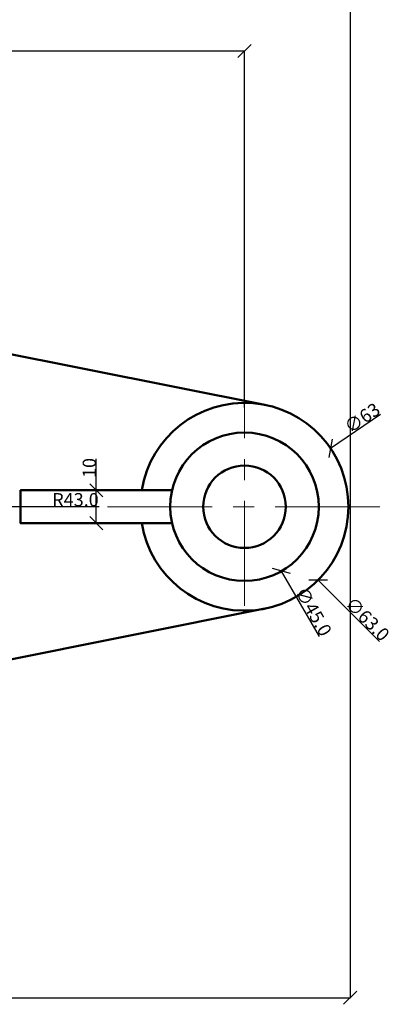
# Model space of a CAD drawing. Units: millimetres. Extents: x 263 to 611, y 50 to 522.
# Tile 4 of 5: x 478 to 591, y 50 to 349. Entities that reach past the tile are written whole.
import ezdxf

# ---------------------------------------------------------------- set-up
doc = ezdxf.new("R2010")
doc.units = ezdxf.units.MM
doc.header["$MEASUREMENT"] = 0
doc.linetypes.add('CENTER', pattern=[50.8, 31.75, -6.35, 6.35, -6.35])
for name, color, linetype, lineweight in [('M-CNTR', 1, 'CENTER', 18), ('M-DIMS', 2, 'Continuous', 25), ('M-OUTL', 7, 'Continuous', 50)]:
    doc.layers.add(name, color=color, linetype=linetype, lineweight=lineweight)
doc.styles.get("Standard").update_dxf_attribs({"font": 'arial.ttf'})
doc.dimstyles.get("Standard").update_dxf_attribs({"dimtxt": 4, "dimasz": 4, "dimexe": 0.18, "dimexo": 0.0625, "dimgap": 0.09, "dimtad": 1, "dimdec": 0, "dimzin": 0, "dimdsep": 46, "dimtxsty": 'Standard', "dimblk": 'OBLIQUE', "dimcen": 0.09, "dimclre": 251, "dimadec": 0, "dimazin": 0, "dimtfac": 1, "dimtdec": 0, "dimtofl": 0, "dimtmove": 0, "dimatfit": 3, "dimfxl": 1, "dimtolj": 1, "dimtzin": 0, "dimarcsym": 0})

# ---------------------------------------------------------------- blocks, each defined once
blk = doc.blocks.new('_Oblique')
at = {"color": 0, "linetype": 'ByBlock', "lineweight": -2}
blk.add_line((-0.5, -0.5), (0.5, 0.5), dxfattribs=at)
blk = doc.blocks.new('*D18')
at = {"layer": 'Defpoints', "color": 0, "transparency": 16777216}
for p in [(546.1, 339.25), (546.1, 231.08), (311.1, 223.08)]:
    blk.add_point(p, dxfattribs=at)
at = {"layer": 'M-DIMS', "color": 0, "lineweight": -2, "transparency": 16777216}
for p, q in [((311.1, 223.14), (311.1, 339.43)), ((311.1, 339.25), (546.1, 339.25)), ((546.1, 231.14), (546.1, 339.43))]:
    blk.add_line(p, q, dxfattribs=at)
at = {"layer": 'M-DIMS', "color": 0, "lineweight": -2, "transparency": 16777216, "xscale": 4, "yscale": 4, "zscale": 4, "rotation": 180}
blk.add_blockref('_Oblique', (311.1, 339.25), dxfattribs=at)
at = {"layer": 'M-DIMS', "color": 0, "lineweight": -2, "transparency": 16777216, "xscale": 4, "yscale": 4, "zscale": 4}
blk.add_blockref('_Oblique', (546.1, 339.25), dxfattribs=at)
at = {"layer": 'M-DIMS', "color": 0, "transparency": 16777216, "insert": (428.6, 341.39), "char_height": 4, "attachment_point": 5}
blk.add_mtext('\\A1;235', dxfattribs=at)
blk = doc.blocks.new('*D28')
at = {"layer": 'Defpoints', "color": 0, "transparency": 16777216}
for p in [(501.21, 206.08), (501.21, 206.08), (501.21, 196.08)]:
    blk.add_point(p, dxfattribs=at)
at = {"layer": 'M-DIMS', "color": 0, "lineweight": -2, "transparency": 16777216}
for p, q in [((501.21, 206.08), (501.21, 215.6)), ((501.15, 206.08), (501.03, 206.08)), ((501.21, 196.08), (501.21, 206.08)), ((501.15, 196.08), (501.03, 196.08))]:
    blk.add_line(p, q, dxfattribs=at)
at = {"layer": 'M-DIMS', "color": 0, "lineweight": -2, "transparency": 16777216, "xscale": 4, "yscale": 4, "zscale": 4}
for p, rotation in [((501.21, 206.08), 90), ((501.21, 196.08), 270)]:
    blk.add_blockref('_Oblique', p, dxfattribs=dict(at, rotation=rotation))
at = {"layer": 'M-DIMS', "color": 0, "transparency": 16777216, "insert": (499.08, 212.84), "char_height": 4, "attachment_point": 5, "rotation": 90}
blk.add_mtext('\\A1;10', dxfattribs=at)
blk = doc.blocks.new('*D34')
at = {"layer": 'Defpoints', "color": 0, "transparency": 16777216}
for p in [(572.16, 218.78), (520.04, 183.39)]:
    blk.add_point(p, dxfattribs=at)
at = {"layer": 'M-DIMS', "color": 0, "lineweight": -2, "transparency": 16777216}
for p, q in [((587.27, 229.04), (572.16, 218.78)), ((546.01, 201.08), (546.19, 201.08)), ((546.1, 200.99), (546.1, 201.17))]:
    blk.add_line(p, q, dxfattribs=at)
at = {"layer": 'M-DIMS', "color": 0, "lineweight": -2, "transparency": 16777216, "xscale": 4, "yscale": 4, "zscale": 4, "rotation": 214.179634482308}
blk.add_blockref('_Oblique', (572.16, 218.78), dxfattribs=at)
at = {"layer": 'M-DIMS', "color": 0, "transparency": 16777216, "insert": (581.76, 228.01), "char_height": 4, "attachment_point": 5, "rotation": 34.1796}
blk.add_mtext('\\A1;∅63', dxfattribs=at)
blk = doc.blocks.new('*D53')
at = {"layer": 'Defpoints', "color": 0, "transparency": 16777216}
for p in [(578.1, 423.27), (311.1, 383.27), (578.1, 52.26)]:
    blk.add_point(p, dxfattribs=at)
at = {"layer": 'M-DIMS', "color": 251, "lineweight": -2, "transparency": 16777216}
for p, q in [((578.1, 423.21), (578.1, 52.08)), ((311.1, 383.21), (311.1, 52.08))]:
    blk.add_line(p, q, dxfattribs=at)
at = {"layer": 'M-DIMS', "color": 0, "lineweight": -2, "transparency": 16777216}
blk.add_line((311.1, 52.26), (578.1, 52.26), dxfattribs=at)
at = {"layer": 'M-DIMS', "color": 0, "lineweight": -2, "transparency": 16777216, "xscale": 4, "yscale": 4, "zscale": 4, "rotation": 180}
blk.add_blockref('_Oblique', (311.1, 52.26), dxfattribs=at)
at = {"layer": 'M-DIMS', "color": 0, "lineweight": -2, "transparency": 16777216, "xscale": 4, "yscale": 4, "zscale": 4}
blk.add_blockref('_Oblique', (578.1, 52.26), dxfattribs=at)
at = {"layer": 'M-DIMS', "color": 0, "transparency": 16777216, "insert": (444.6, 54.39), "char_height": 4, "attachment_point": 5}
blk.add_mtext('\\A1;267.0', dxfattribs=at)
blk = doc.blocks.new('*D70')
at = {"layer": 'Defpoints', "color": 0, "transparency": 16777216}
for p in [(426.1, 201.08), (469.1, 201.08)]:
    blk.add_point(p, dxfattribs=at)
at = {"layer": 'M-DIMS', "color": 251, "lineweight": -2, "transparency": 16777216}
for p, q in [((426.01, 201.08), (426.19, 201.08)), ((426.1, 200.99), (426.1, 201.17))]:
    blk.add_line(p, q, dxfattribs=at)
at = {"layer": 'M-DIMS', "color": 0, "lineweight": -2, "transparency": 16777216}
blk.add_line((502.09, 201.08), (469.1, 201.08), dxfattribs=at)
at = {"layer": 'M-DIMS', "color": 0, "lineweight": -2, "transparency": 16777216, "xscale": 4, "yscale": 4, "zscale": 4, "rotation": 180.0006262561947}
blk.add_blockref('_Oblique', (469.1, 201.08), dxfattribs=at)
at = {"layer": 'M-DIMS', "color": 0, "transparency": 16777216, "insert": (494.9, 203.22), "char_height": 4, "attachment_point": 5, "rotation": 0.0006}
blk.add_mtext('\\A1;R43.0', dxfattribs=at)
blk = doc.blocks.new('*D72')
at = {"layer": 'Defpoints', "color": 0, "transparency": 16777216}
for p in [(523.82, 223.35), (568.38, 178.82)]:
    blk.add_point(p, dxfattribs=at)
at = {"layer": 'M-DIMS', "color": 251, "lineweight": -2, "transparency": 16777216}
for p, q in [((546.01, 201.08), (546.19, 201.08)), ((546.1, 200.99), (546.1, 201.17))]:
    blk.add_line(p, q, dxfattribs=at)
at = {"layer": 'M-DIMS', "color": 0, "lineweight": -2, "transparency": 16777216}
blk.add_line((587.03, 160.19), (568.38, 178.82), dxfattribs=at)
at = {"layer": 'M-DIMS', "color": 0, "lineweight": -2, "transparency": 16777216, "xscale": 4, "yscale": 4, "zscale": 4, "rotation": 135.0252345814981}
blk.add_blockref('_Oblique', (568.38, 178.82), dxfattribs=at)
at = {"layer": 'M-DIMS', "color": 0, "transparency": 16777216, "insert": (583.34, 167.05), "char_height": 4, "attachment_point": 5, "rotation": 315.0252}
blk.add_mtext('\\A1;∅63.0', dxfattribs=at)
blk = doc.blocks.new('*D73')
at = {"layer": 'Defpoints', "color": 0, "transparency": 16777216}
for p in [(534.85, 220.57), (557.35, 181.59)]:
    blk.add_point(p, dxfattribs=at)
at = {"layer": 'M-DIMS', "color": 251, "lineweight": -2, "transparency": 16777216}
for p, q in [((546.01, 201.08), (546.19, 201.08)), ((546.1, 200.99), (546.1, 201.17))]:
    blk.add_line(p, q, dxfattribs=at)
at = {"layer": 'M-DIMS', "color": 0, "lineweight": -2, "transparency": 16777216}
blk.add_line((568.8, 161.75), (557.35, 181.59), dxfattribs=at)
at = {"layer": 'M-DIMS', "color": 0, "lineweight": -2, "transparency": 16777216, "xscale": 4, "yscale": 4, "zscale": 4, "rotation": 119.9949843356095}
blk.add_blockref('_Oblique', (557.35, 181.59), dxfattribs=at)
at = {"layer": 'M-DIMS', "color": 0, "transparency": 16777216, "insert": (567.02, 169.33), "char_height": 4, "attachment_point": 5, "rotation": 299.995}
blk.add_mtext('\\A1;∅45.0', dxfattribs=at)

msp = doc.modelspace()

# ---------------------------------------------------------------- linework, layer by layer
at = {"layer": 'M-CNTR'}
for p, q in [((546.0988, 171.0815), (546.0988, 231.0815)), ((587.1329, 201.0815), (311.0988, 201.0815))]:
    msp.add_line(p, q, dxfattribs=at)
at = {"layer": 'M-OUTL'}
for p, q in [((552.2661, 231.9719), (436.0988, 255.1648)), ((552.2661, 170.1912), (436.0988, 146.9983))]:
    msp.add_line(p, q, dxfattribs=at)
msp.add_lwpolyline([(524.1614, 196.0815), (478.2588, 196.0815), (478.2588, 206.0815), (524.1614, 206.0815)], dxfattribs=at)
for radius in [22.5, 12.5]:
    msp.add_circle((546.0988, 201.0815), radius, dxfattribs=at)
msp.add_arc((546.0988, 201.0815), 31.5, 189.133198, 170.866802, dxfattribs=at)

# ---------------------------------------------------------------- dimensions: what is measured, and where the dimension line sits
at = {"layer": 'M-DIMS'}
for base, p1, p2, override, picture, middle in [((578.0988, 52.2557), (311.0988, 383.2727), (578.0988, 423.2727), {"dimdec": 1, "dimlfac": 1, "dimrnd": 0, "dimzin": 0, "dimdsep": 46, "dimlunit": 2}, '*D53', (444.5988, 54.388)), ((546.0988, 339.2528), (311.0988, 223.0815), (546.0988, 231.0815), {"dimclrd": 0, "dimclre": 0, "dimclrt": 0}, '*D18', (428.5988, 341.3864))]:
    dim = msp.add_linear_dim(base=base, p1=p1, p2=p2, dimstyle='Standard', override=override, dxfattribs=at)
    dim.commit()
    dim.dimension.update_dxf_attribs({"geometry": picture, "text_midpoint": middle})
dim = msp.add_diameter_dim_2p(p1=(520.0395, 183.3852), p2=(572.1582, 218.7779), dimstyle='Standard', override={"dimclrd": 0, "dimclre": 0, "dimclrt": 0}, dxfattribs=at)
dim.commit()
dim.dimension.update_dxf_attribs({"geometry": '*D34', "text_midpoint": (581.7604, 228.0113)})
for p1, p2, picture, middle in [((523.8152, 223.3456), (568.3825, 178.8175), '*D72', (581.7527, 165.459)), ((534.8505, 220.5681), (557.3471, 181.595), '*D73', (565.0731, 168.2105))]:
    dim = msp.add_diameter_dim_2p(p1=p1, p2=p2, dimstyle='Standard', override={"dimdec": 1, "dimlfac": 1, "dimrnd": 0, "dimzin": 0, "dimdsep": 46, "dimlunit": 2}, dxfattribs=at)
    dim.commit()
    dim.dimension.update_dxf_attribs({"geometry": picture, "text_midpoint": middle, "dimtype": 163})
dim = msp.add_linear_dim(base=(501.2101, 206.0815), p1=(501.2101, 196.0815), p2=(501.2101, 206.0815), angle=90, dimstyle='Standard', override={"dimclrd": 0, "dimclre": 0, "dimclrt": 0}, dxfattribs=at)
dim.commit()
dim.dimension.update_dxf_attribs({"geometry": '*D28', "text_midpoint": (501.2101, 212.8414), "dimtype": 160})
dim = msp.add_radius_dim(center=(426.0988, 201.0815), mpoint=(469.0988, 201.082), dimstyle='Standard', override={"dimdec": 1, "dimlfac": 1, "dimrnd": 0, "dimzin": 0, "dimdsep": 46, "dimlunit": 2}, dxfattribs=at)
dim.commit()
dim.dimension.update_dxf_attribs({"geometry": '*D70', "text_midpoint": (494.8988, 201.0823), "dimtype": 164})

doc.saveas('drawing.dxf')
